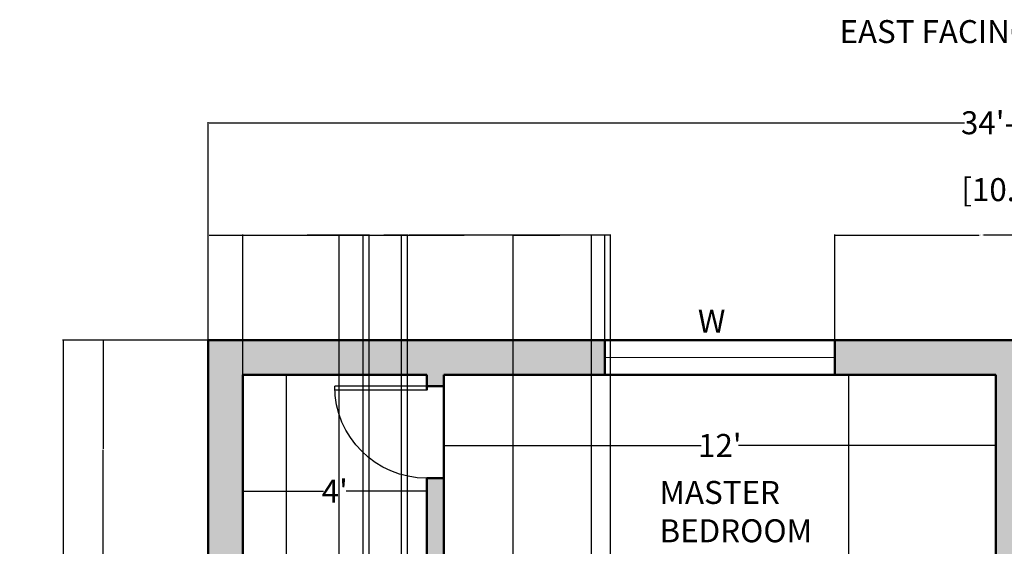
# Model space of a CAD drawing. Units: inches. Extents: x -22 to 470, y -437 to 97.
# Tile 7 of 9: x -22 to 235, y -41 to 97. Entities that reach past the tile are written whole.
import ezdxf

# ---------------------------------------------------------------- set-up
doc = ezdxf.new("R2010")
doc.units = ezdxf.units.IN
doc.header["$MEASUREMENT"] = 0
for name, color, linetype, lineweight in [('A-ANNO-DIMS', 2, 'Continuous', 18), ('A-ANNO-TEXT', 7, 'Continuous', 18), ('A-AREA-IDEN', 7, 'Continuous', 25), ('A-DOOR', 4, 'Continuous', 25), ('A-GLAZ', 4, 'Continuous', 18), ('A-WALL', 7, 'Continuous', 50), ('A-WALL-PATT', 8, 'Continuous', 13)]:
    doc.layers.add(name, color=color, linetype=linetype, lineweight=lineweight)
doc.styles.get("Standard").update_dxf_attribs({"font": 'arial.ttf'})
doc.dimstyles.get("Standard").update_dxf_attribs({"dimtxt": 0.18, "dimasz": 0.18, "dimexe": 0.18, "dimexo": 0.0625, "dimgap": 0.09, "dimtad": 0, "dimtih": 1, "dimtoh": 1, "dimdec": 0, "dimzin": 0, "dimdsep": 46, "dimlunit": 3, "dimtxsty": 'Standard', "dimcen": 0.09, "dimadec": 0, "dimazin": 0, "dimtfac": 1, "dimtdec": 0, "dimtofl": 0, "dimtmove": 0, "dimatfit": 3, "dimfxl": 1, "dimtolj": 1, "dimtzin": 0, "dimarcsym": 0})

# ---------------------------------------------------------------- blocks, each defined once
blk = doc.blocks.new('*D2')
at = {"layer": 'A-ANNO-DIMS', "color": 0, "lineweight": -2, "transparency": 16777216}
for p, q in [((26.92, 13.31), (26.92, 70.17)), ((27.1, 69.99), (224.28, 69.99)), ((442.24, 69.99), (245.07, 69.99)), ((442.42, 13.31), (442.42, 70.17))]:
    blk.add_line(p, q, dxfattribs=at)
at = {"layer": 'A-ANNO-DIMS', "color": 0, "transparency": 16777216}
for points in [[(27.1, 70.02), (27.1, 69.96), (26.92, 69.99)], [(442.24, 70.02), (442.24, 69.96), (442.42, 69.99)]]:
    blk.add_solid(points, dxfattribs=at)
at = {"layer": 'Defpoints', "color": 0, "transparency": 16777216}
for p in [(442.42, 69.99), (26.92, 13.24), (442.42, 13.24)]:
    blk.add_point(p, dxfattribs=at)
at = {"layer": 'A-ANNO-DIMS', "color": 0, "transparency": 16777216, "insert": (234.67, 69.99), "char_height": 6, "attachment_point": 5}
blk.add_mtext('\\A1;34\'-8"', dxfattribs=at)
blk = doc.blocks.new('*D3')
at = {"layer": 'A-ANNO-DIMS', "color": 0, "lineweight": -2, "transparency": 16777216}
for p, q in [((26.86, 13.24), (-11.18, 13.24)), ((-11, 13.06), (-11, -189.1)), ((-11, -397.58), (-11, -195.41)), ((26.86, -397.76), (-11.18, -397.76))]:
    blk.add_line(p, q, dxfattribs=at)
at = {"layer": 'A-ANNO-DIMS', "color": 0, "transparency": 16777216}
for points in [[(-11.03, 13.06), (-10.97, 13.06), (-11, 13.24)], [(-11.03, -397.58), (-10.97, -397.58), (-11, -397.76)]]:
    blk.add_solid(points, dxfattribs=at)
at = {"layer": 'Defpoints', "color": 0, "transparency": 16777216}
for p in [(26.92, 13.24), (-11, -397.76), (26.92, -397.76)]:
    blk.add_point(p, dxfattribs=at)
at = {"layer": 'A-ANNO-DIMS', "color": 0, "transparency": 16777216, "insert": (-11, -192.26), "char_height": 6, "attachment_point": 5}
blk.add_mtext('\\A1;34\'-3"', dxfattribs=at)
blk = doc.blocks.new('*D4')
at = {"layer": 'A-ANNO-DIMS', "color": 0, "lineweight": -2, "transparency": 16777216}
for p, q in [((35.92, -27.85), (35.92, -25.95)), ((36.1, -26.13), (56.95, -26.13)), ((83.74, -26.13), (62.89, -26.13)), ((83.92, -27.85), (83.92, -25.95))]:
    blk.add_line(p, q, dxfattribs=at)
at = {"layer": 'A-ANNO-DIMS', "color": 0, "transparency": 16777216}
for points in [[(36.1, -26.1), (36.1, -26.16), (35.92, -26.13)], [(83.74, -26.1), (83.74, -26.16), (83.92, -26.13)]]:
    blk.add_solid(points, dxfattribs=at)
at = {"layer": 'Defpoints', "color": 0, "transparency": 16777216}
for p in [(35.92, -26.13), (35.92, -27.91), (83.92, -27.91)]:
    blk.add_point(p, dxfattribs=at)
at = {"layer": 'A-ANNO-DIMS', "color": 0, "transparency": 16777216, "insert": (59.92, -26.13), "char_height": 6, "attachment_point": 5}
blk.add_mtext("\\A1;4'", dxfattribs=at)
blk = doc.blocks.new('*D5')
at = {"layer": 'A-ANNO-DIMS', "color": 0, "lineweight": -2, "transparency": 16777216}
for p, q in [((47.18, 4.24), (47.06, 4.24)), ((47.24, 4.06), (47.24, -52.6)), ((47.24, -115.58), (47.24, -58.91)), ((47.18, -115.76), (47.06, -115.76))]:
    blk.add_line(p, q, dxfattribs=at)
at = {"layer": 'A-ANNO-DIMS', "color": 0, "transparency": 16777216}
for points in [[(47.21, 4.06), (47.27, 4.06), (47.24, 4.24)], [(47.21, -115.58), (47.27, -115.58), (47.24, -115.76)]]:
    blk.add_solid(points, dxfattribs=at)
at = {"layer": 'Defpoints', "color": 0, "transparency": 16777216}
for p in [(47.24, 4.24), (47.24, 4.24), (47.24, -115.76)]:
    blk.add_point(p, dxfattribs=at)
at = {"layer": 'A-ANNO-DIMS', "color": 0, "transparency": 16777216, "insert": (47.24, -55.76), "char_height": 6, "attachment_point": 5}
blk.add_mtext("\\A1;10'", dxfattribs=at)
blk = doc.blocks.new('*D6')
at = {"layer": 'A-ANNO-DIMS', "color": 0, "lineweight": -2, "transparency": 16777216}
for p, q in [((194.01, 4.06), (194.01, -52.6)), ((194.07, 4.24), (194.19, 4.24)), ((194.01, -115.58), (194.01, -58.91)), ((194.07, -115.76), (194.19, -115.76))]:
    blk.add_line(p, q, dxfattribs=at)
at = {"layer": 'A-ANNO-DIMS', "color": 0, "transparency": 16777216}
for points in [[(193.98, 4.06), (194.04, 4.06), (194.01, 4.24)], [(193.98, -115.58), (194.04, -115.58), (194.01, -115.76)]]:
    blk.add_solid(points, dxfattribs=at)
at = {"layer": 'Defpoints', "color": 0, "transparency": 16777216}
for p in [(194.01, 4.24), (194.01, 4.24), (194.01, -115.76)]:
    blk.add_point(p, dxfattribs=at)
at = {"layer": 'A-ANNO-DIMS', "color": 0, "transparency": 16777216, "insert": (194.01, -55.76), "char_height": 6, "attachment_point": 5}
blk.add_mtext("\\A1;10'", dxfattribs=at)
blk = doc.blocks.new('*D7')
at = {"layer": 'A-ANNO-DIMS', "color": 0, "lineweight": -2, "transparency": 16777216}
for p, q in [((88.42, -14.46), (88.42, -14.04)), ((88.6, -14.22), (155.52, -14.22)), ((232.24, -14.22), (165.32, -14.22)), ((232.42, -14.46), (232.42, -14.04))]:
    blk.add_line(p, q, dxfattribs=at)
at = {"layer": 'A-ANNO-DIMS', "color": 0, "transparency": 16777216}
for points in [[(88.6, -14.19), (88.6, -14.25), (88.42, -14.22)], [(232.24, -14.19), (232.24, -14.25), (232.42, -14.22)]]:
    blk.add_solid(points, dxfattribs=at)
at = {"layer": 'Defpoints', "color": 0, "transparency": 16777216}
for p in [(88.42, -14.22), (88.42, -14.52), (232.42, -14.52)]:
    blk.add_point(p, dxfattribs=at)
at = {"layer": 'A-ANNO-DIMS', "color": 0, "transparency": 16777216, "insert": (160.42, -14.22), "char_height": 6, "attachment_point": 5}
blk.add_mtext("\\A1;12'", dxfattribs=at)
blk = doc.blocks.new('DOOR-SWING-24')
for p, q in [((23, 24), (23, 0)), ((24, 24), (24, 0))]:
    blk.add_line(p, q)
blk.add_arc((24, 24), 24, 180, 270)
blk = doc.blocks.new('WINDOW-60-SASH')
for p, q in [((0, 9), (60, 9)), ((0, 4.5), (60, 4.5)), ((60, 0), (0, 0))]:
    blk.add_line(p, q)
blk = doc.blocks.new('*D63')
at = {"layer": 'A-ANNO-DIMS', "color": 0, "lineweight": -2, "transparency": 16777216}
for p, q in [((68.92, -120.19), (68.92, 40.87)), ((69.1, 40.69), (73.52, 40.69)), ((78.74, 40.69), (74.32, 40.69)), ((78.92, -120.19), (78.92, 40.87))]:
    blk.add_line(p, q, dxfattribs=at)
at = {"layer": 'A-ANNO-DIMS', "color": 0, "transparency": 16777216}
for points in [[(69.1, 40.72), (69.1, 40.66), (68.92, 40.69)], [(78.74, 40.72), (78.74, 40.66), (78.92, 40.69)]]:
    blk.add_solid(points, dxfattribs=at)
at = {"layer": 'Defpoints', "color": 0, "transparency": 16777216}
for p in [(78.92, 40.69), (68.92, -120.26), (78.92, -120.26)]:
    blk.add_point(p, dxfattribs=at)
at = {"layer": 'A-ANNO-DIMS', "color": 0, "transparency": 16777216, "insert": (73.92, 40.69), "char_height": 0.18, "attachment_point": 5}
blk.add_mtext('\\A1;0\'-10"', dxfattribs=at)
blk = doc.blocks.new('*D65')
at = {"layer": 'A-ANNO-DIMS', "color": 0, "lineweight": -2, "transparency": 16777216}
for p, q in [((26.92, 13.31), (26.92, 40.87)), ((27.1, 40.69), (78.13, 40.69)), ((130.24, 40.69), (79.21, 40.69)), ((130.42, 13.31), (130.42, 40.87))]:
    blk.add_line(p, q, dxfattribs=at)
at = {"layer": 'A-ANNO-DIMS', "color": 0, "transparency": 16777216}
for points in [[(27.1, 40.72), (27.1, 40.66), (26.92, 40.69)], [(130.24, 40.72), (130.24, 40.66), (130.42, 40.69)]]:
    blk.add_solid(points, dxfattribs=at)
at = {"layer": 'Defpoints', "color": 0, "transparency": 16777216}
for p in [(130.42, 40.69), (26.92, 13.24), (130.42, 13.24)]:
    blk.add_point(p, dxfattribs=at)
at = {"layer": 'A-ANNO-DIMS', "color": 0, "transparency": 16777216, "insert": (78.67, 40.69), "char_height": 0.18, "attachment_point": 5}
blk.add_mtext('\\A1;8\'-7 1/2"', dxfattribs=at)
blk = doc.blocks.new('*D66')
at = {"layer": 'A-ANNO-DIMS', "color": 0, "lineweight": -2, "transparency": 16777216}
for p, q in [((190.42, 13.31), (190.42, 40.87)), ((190.6, 40.69), (228.13, 40.69)), ((266.74, 40.69), (229.21, 40.69)), ((266.92, 13.31), (266.92, 40.87))]:
    blk.add_line(p, q, dxfattribs=at)
at = {"layer": 'A-ANNO-DIMS', "color": 0, "transparency": 16777216}
for points in [[(190.6, 40.72), (190.6, 40.66), (190.42, 40.69)], [(266.74, 40.72), (266.74, 40.66), (266.92, 40.69)]]:
    blk.add_solid(points, dxfattribs=at)
at = {"layer": 'Defpoints', "color": 0, "transparency": 16777216}
for p in [(266.92, 40.69), (190.42, 13.24), (266.92, 13.24)]:
    blk.add_point(p, dxfattribs=at)
at = {"layer": 'A-ANNO-DIMS', "color": 0, "transparency": 16777216, "insert": (228.67, 40.69), "char_height": 0.18, "attachment_point": 5}
blk.add_mtext('\\A1;6\'-4 1/2"', dxfattribs=at)
blk = doc.blocks.new('*D67')
at = {"layer": 'A-ANNO-DIMS', "color": 0, "lineweight": -2, "transparency": 16777216}
for p, q in [((26.86, 13.24), (-0.71, 13.24)), ((-0.53, 13.06), (-0.53, -15.07)), ((-0.53, -43.58), (-0.53, -15.44)), ((26.86, -43.76), (-0.71, -43.76))]:
    blk.add_line(p, q, dxfattribs=at)
at = {"layer": 'A-ANNO-DIMS', "color": 0, "transparency": 16777216}
for points in [[(-0.56, 13.06), (-0.5, 13.06), (-0.53, 13.24)], [(-0.56, -43.58), (-0.5, -43.58), (-0.53, -43.76)]]:
    blk.add_solid(points, dxfattribs=at)
at = {"layer": 'Defpoints', "color": 0, "transparency": 16777216}
for p in [(26.92, 13.24), (-0.53, -43.76), (26.92, -43.76)]:
    blk.add_point(p, dxfattribs=at)
at = {"layer": 'A-ANNO-DIMS', "color": 0, "transparency": 16777216, "insert": (-0.53, -15.26), "char_height": 0.18, "attachment_point": 5}
blk.add_mtext('\\A1;4\'-9"', dxfattribs=at)
blk = doc.blocks.new('*D78')
at = {"layer": 'A-ANNO-DIMS', "color": 0, "lineweight": -2, "transparency": 16777216}
for p, q in [((35.92, -192.19), (35.92, 40.87)), ((36.1, 40.69), (52.09, 40.69)), ((68.74, 40.69), (52.75, 40.69)), ((68.92, -192.19), (68.92, 40.87))]:
    blk.add_line(p, q, dxfattribs=at)
at = {"layer": 'A-ANNO-DIMS', "color": 0, "transparency": 16777216}
for points in [[(36.1, 40.72), (36.1, 40.66), (35.92, 40.69)], [(68.74, 40.72), (68.74, 40.66), (68.92, 40.69)]]:
    blk.add_solid(points, dxfattribs=at)
at = {"layer": 'Defpoints', "color": 0, "transparency": 16777216}
for p in [(68.92, 40.69), (35.92, -192.26), (68.92, -192.26)]:
    blk.add_point(p, dxfattribs=at)
at = {"layer": 'A-ANNO-DIMS', "color": 0, "transparency": 16777216, "insert": (52.42, 40.69), "char_height": 0.18, "attachment_point": 5}
blk.add_mtext('\\A1;2\'-9"', dxfattribs=at)
blk = doc.blocks.new('*D79')
at = {"layer": 'A-ANNO-DIMS', "color": 0, "lineweight": -2, "transparency": 16777216}
for p, q in [((61.08, -228.48), (61.08, 40.87)), ((61.26, 40.69), (93.66, 40.69)), ((126.72, 40.69), (94.32, 40.69)), ((126.9, -228.48), (126.9, 40.87))]:
    blk.add_line(p, q, dxfattribs=at)
at = {"layer": 'A-ANNO-DIMS', "color": 0, "transparency": 16777216}
for points in [[(61.26, 40.72), (61.26, 40.66), (61.08, 40.69)], [(126.72, 40.72), (126.72, 40.66), (126.9, 40.69)]]:
    blk.add_solid(points, dxfattribs=at)
at = {"layer": 'Defpoints', "color": 0, "transparency": 16777216}
for p in [(126.9, 40.69), (61.08, -228.55), (126.9, -228.55)]:
    blk.add_point(p, dxfattribs=at)
at = {"layer": 'A-ANNO-DIMS', "color": 0, "transparency": 16777216, "insert": (93.99, 40.69), "char_height": 0.18, "attachment_point": 5}
blk.add_mtext('\\A1;5\'-6"', dxfattribs=at)
blk = doc.blocks.new('*D83')
at = {"layer": 'A-ANNO-DIMS', "color": 0, "lineweight": -2, "transparency": 16777216}
for p, q in [((67.35, -370.26), (67.35, 40.87)), ((67.53, 40.69), (71.94, 40.69)), ((77.15, 40.69), (72.74, 40.69)), ((77.33, -369.14), (77.33, 40.87))]:
    blk.add_line(p, q, dxfattribs=at)
at = {"layer": 'A-ANNO-DIMS', "color": 0, "transparency": 16777216}
for points in [[(67.53, 40.72), (67.53, 40.66), (67.35, 40.69)], [(77.15, 40.72), (77.15, 40.66), (77.33, 40.69)]]:
    blk.add_solid(points, dxfattribs=at)
at = {"layer": 'Defpoints', "color": 0, "transparency": 16777216}
for p in [(77.33, 40.69), (77.33, -369.2), (67.35, -370.32)]:
    blk.add_point(p, dxfattribs=at)
at = {"layer": 'A-ANNO-DIMS', "color": 0, "transparency": 16777216, "insert": (72.34, 40.69), "char_height": 0.18, "attachment_point": 5}
blk.add_mtext('\\A1;0\'-10"', dxfattribs=at)
blk = doc.blocks.new('*D84')
at = {"layer": 'A-ANNO-DIMS', "color": 0, "lineweight": -2, "transparency": 16777216}
for p, q in [((106.48, -369.14), (106.48, 40.87)), ((106.66, 40.69), (118.66, 40.69)), ((131.74, 40.69), (119.74, 40.69)), ((131.92, -388.69), (131.92, 40.87))]:
    blk.add_line(p, q, dxfattribs=at)
at = {"layer": 'A-ANNO-DIMS', "color": 0, "transparency": 16777216}
for points in [[(106.66, 40.72), (106.66, 40.66), (106.48, 40.69)], [(131.74, 40.72), (131.74, 40.66), (131.92, 40.69)]]:
    blk.add_solid(points, dxfattribs=at)
at = {"layer": 'Defpoints', "color": 0, "transparency": 16777216}
for p in [(131.92, 40.69), (106.48, -369.2), (131.92, -388.76)]:
    blk.add_point(p, dxfattribs=at)
at = {"layer": 'A-ANNO-DIMS', "color": 0, "transparency": 16777216, "insert": (119.2, 40.69), "char_height": 0.18, "attachment_point": 5}
blk.add_mtext('\\A1;2\'-1 1/2"', dxfattribs=at)

msp = doc.modelspace()

# ---------------------------------------------------------------- hatches: boundary and pattern name
at = {"layer": 'A-WALL-PATT'}
h = msp.add_hatch(color=256, dxfattribs=at)
h.dxf.hatch_style = 1
h.paths.add_polyline_path([(130.42, 13.24), (26.92, 13.24), (26.92, -43.76), (35.92, -43.76), (35.92, 4.24), (83.92, 4.24), (83.92, 1.24), (88.42, 1.24), (88.42, 4.24), (130.42, 4.24)])
h.paths.add_polyline_path([(266.92, 13.24), (190.42, 13.24), (190.42, 4.24), (232.42, 4.24), (232.42, -115.76), (229.42, -115.76), (229.42, -120.26), (239.92, -120.26), (239.92, -115.76), (236.92, -115.76), (236.92, 4.24), (266.92, 4.24)])
h.paths.add_polyline_path([(442.42, 13.24), (326.92, 13.24), (326.92, 4.24), (356.92, 4.24), (356.92, 1.24), (361.42, 1.24), (361.42, 4.24), (433.42, 4.24), (433.42, -49.38), (442.42, -49.38)])
h.paths.add_polyline_path([(442.42, -73.38), (433.42, -73.38), (433.42, -115.76), (361.42, -115.76), (361.42, -22.76), (356.92, -22.76), (356.92, -115.76), (263.92, -115.76), (263.92, -120.26), (332.92, -120.26), (332.92, -123.26), (337.42, -123.26), (337.42, -120.26), (433.42, -120.26), (433.42, -148.49), (442.42, -148.49)])
h.paths.add_polyline_path([(205.42, -115.76), (88.42, -115.76), (88.42, -22.76), (83.92, -22.76), (83.92, -115.76), (35.92, -115.76), (35.92, -67.76), (26.92, -67.76), (26.92, -126.26), (35.92, -126.26), (35.92, -120.26), (205.42, -120.26)])
h.paths.add_polyline_path([(35.92, -196.76), (168.92, -196.76), (168.92, -192.26), (35.92, -192.26), (35.92, -186.26), (26.92, -186.26), (26.92, -224.25), (35.92, -224.25)])
h.paths.add_polyline_path([(35.92, -284.25), (26.92, -284.25), (26.92, -397.76), (53.92, -397.76), (53.92, -388.76), (35.92, -388.76)])
h.paths.add_polyline_path([(142.42, -388.76), (136.42, -388.76), (136.42, -316.76), (181.42, -316.76), (181.42, -312.26), (136.42, -312.26), (136.42, -303.75), (131.92, -303.75), (131.92, -388.76), (113.92, -388.76), (113.92, -397.76), (142.42, -397.76)])
h.paths.add_polyline_path([(218.92, -388.76), (212.92, -388.76), (212.92, -312.26), (205.42, -312.26), (205.42, -316.76), (208.42, -316.76), (208.42, -388.76), (202.42, -388.76), (202.42, -397.76), (218.92, -397.76)])
h.paths.add_polyline_path([(306.75, -388.76), (289.42, -388.76), (289.42, -316.76), (284.92, -316.76), (284.92, -388.76), (278.92, -388.76), (278.92, -397.76), (306.75, -397.76)])
h.paths.add_polyline_path([(391.42, -388.76), (366.75, -388.76), (366.75, -397.76), (391.42, -397.76)], flags=17)
h.paths.add_polyline_path([(442.42, -172.49), (433.42, -172.49), (433.42, -192.26), (337.42, -192.26), (337.42, -147.26), (332.92, -147.26), (332.92, -196.76), (433.42, -196.76), (433.42, -388.76), (427.42, -388.76), (427.42, -397.76), (442.42, -397.76)])

# ---------------------------------------------------------------- linework, layer by layer
at = {"layer": 'A-WALL'}
for p, q in [((26.92, 13.24), (26.92, -397.76)), ((26.92, 13.24), (442.42, 13.24)), ((130.42, 4.24), (130.42, 13.24)), ((190.42, 13.24), (190.42, 4.24)), ((35.92, 4.24), (83.92, 4.24)), ((35.92, 4.24), (35.92, -115.76)), ((83.92, 4.24), (83.92, 0.24)), ((88.42, 4.24), (88.42, -115.76)), ((88.42, 4.24), (232.42, 4.24)), ((232.42, 4.24), (232.42, -115.76)), ((88.42, 1.24), (83.92, 1.24)), ((88.42, -22.76), (83.92, -22.76)), ((83.92, -22.76), (83.92, -115.76))]:
    msp.add_line(p, q, dxfattribs=at)

# ---------------------------------------------------------------- block references
at = {"layer": 'A-DOOR', "extrusion": (0, 0, -1), "zscale": -1, "rotation": 89.99999999999989}
msp.add_blockref('DOOR-SWING-24', (-59.92, -22.76), dxfattribs=at)
at = {"layer": 'A-GLAZ'}
msp.add_blockref('WINDOW-60-SASH', (130.42, 4.24), dxfattribs=at)

# ---------------------------------------------------------------- texts
at = {"layer": 'A-ANNO-DIMS', "insert": (223.46, 55.54), "char_height": 6, "attachment_point": 1}
msp.add_mtext_dynamic_manual_height_columns('[10.67]', width=2.641, gutter_width=1, heights=[0], dxfattribs=at)
at = {"layer": 'A-ANNO-TEXT', "char_height": 6, "attachment_point": 1}
for s, insert in [('EAST FACING HOUSE', (191.66, 96.78)), ('W', (154.69, 21.23))]:
    msp.add_mtext(s, dxfattribs=dict(at, insert=insert))
at = {"layer": 'A-AREA-IDEN', "insert": (144.68, -23.48), "char_height": 6, "attachment_point": 1}
msp.add_mtext('MASTER\\PBEDROOM', dxfattribs=at)

# ---------------------------------------------------------------- dimensions: what is measured, and where the dimension line sits
at = {"layer": 'A-ANNO-DIMS'}
for base, p1, p2, override, picture, middle in [((442.42161427, 69.98621919), (26.92161427, 13.24363331), (442.42161427, 13.24363331), {"dimtxt": 6, "dimclrd": 0, "dimclre": 0, "dimclrt": 0}, '*D2', (234.67161427, 69.98621919)), ((130.42, 40.69), (26.92, 13.24), (130.42, 13.24), {"dimdec": 1, "dimlfac": 1, "dimrnd": 0, "dimzin": 1, "dimdsep": 46, "dimlunit": 4, "dimfrac": 2}, '*D65', (78.67, 40.69)), ((68.92, 40.69), (35.92, -192.26), (68.92, -192.26), {"dimdec": 1, "dimlfac": 1, "dimrnd": 0, "dimzin": 1, "dimdsep": 46, "dimlunit": 4, "dimfrac": 2}, '*D78', (52.42, 40.69)), ((126.9, 40.69), (61.08, -228.55), (126.9, -228.55), {"dimdec": 1, "dimlfac": 1, "dimrnd": 0, "dimzin": 1, "dimdsep": 46, "dimlunit": 4, "dimfrac": 2}, '*D79', (93.99, 40.69)), ((77.33, 40.69), (67.35, -370.32), (77.33, -369.2), {"dimdec": 1, "dimlfac": 1, "dimrnd": 0, "dimzin": 1, "dimdsep": 46, "dimlunit": 4, "dimfrac": 2}, '*D83', (72.34, 40.69)), ((78.92, 40.69), (68.92, -120.26), (78.92, -120.26), {"dimdec": 1, "dimlfac": 1, "dimrnd": 0, "dimzin": 1, "dimdsep": 46, "dimlunit": 4, "dimfrac": 2}, '*D63', (73.92, 40.69)), ((131.92, 40.69), (106.48, -369.2), (131.92, -388.76), {"dimdec": 1, "dimlfac": 1, "dimrnd": 0, "dimzin": 1, "dimdsep": 46, "dimlunit": 4, "dimfrac": 2}, '*D84', (119.2, 40.69)), ((266.92, 40.69), (190.42, 13.24), (266.92, 13.24), {"dimdec": 1, "dimlfac": 1, "dimrnd": 0, "dimzin": 1, "dimdsep": 46, "dimlunit": 4, "dimfrac": 2}, '*D66', (228.67, 40.69)), ((88.42, -14.22), (232.42, -14.52), (88.42, -14.52), {"dimtxt": 6, "dimclrd": 0, "dimclre": 0, "dimclrt": 0}, '*D7', (160.42, -14.22)), ((35.92, -26.13), (83.92, -27.91), (35.92, -27.91), {"dimtxt": 6, "dimclrd": 0, "dimclre": 0, "dimclrt": 0}, '*D4', (59.92, -26.13))]:
    dim = msp.add_linear_dim(base=base, p1=p1, p2=p2, dimstyle='Standard', override=override, dxfattribs=at)
    dim.commit()
    dim.dimension.update_dxf_attribs({"geometry": picture, "text_midpoint": middle})
for base, p1, p2, override, picture, middle in [((-11, -397.76), (26.92, 13.24), (26.92, -397.76), {"dimtxt": 6, "dimclrd": 0, "dimclre": 0, "dimclrt": 0}, '*D3', (-11, -192.26)), ((-0.53, -43.76), (26.92, 13.24), (26.92, -43.76), {"dimdec": 1, "dimlfac": 1, "dimrnd": 0, "dimzin": 1, "dimdsep": 46, "dimlunit": 4, "dimfrac": 2}, '*D67', (-0.53, -15.26)), ((47.24, 4.24), (47.24, -115.76), (47.24, 4.24), {"dimtxt": 6, "dimclrd": 0, "dimclre": 0, "dimclrt": 0}, '*D5', (47.24, -55.76)), ((194.01, 4.24), (194.01, -115.76), (194.01, 4.24), {"dimtxt": 6, "dimclrd": 0, "dimclre": 0, "dimclrt": 0}, '*D6', (194.01, -55.76))]:
    dim = msp.add_linear_dim(base=base, p1=p1, p2=p2, angle=90, dimstyle='Standard', override=override, dxfattribs=at)
    dim.commit()
    dim.dimension.update_dxf_attribs({"geometry": picture, "text_midpoint": middle})

doc.saveas('drawing.dxf')
